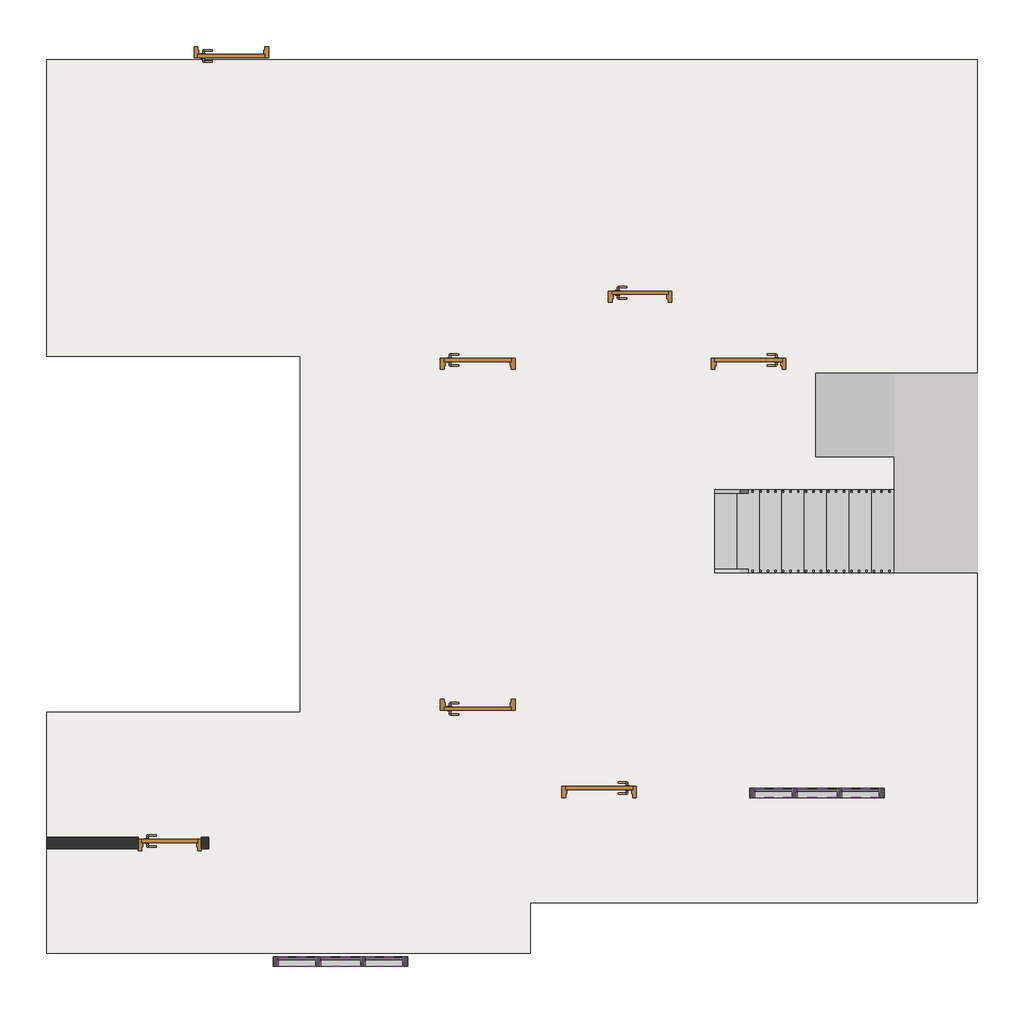
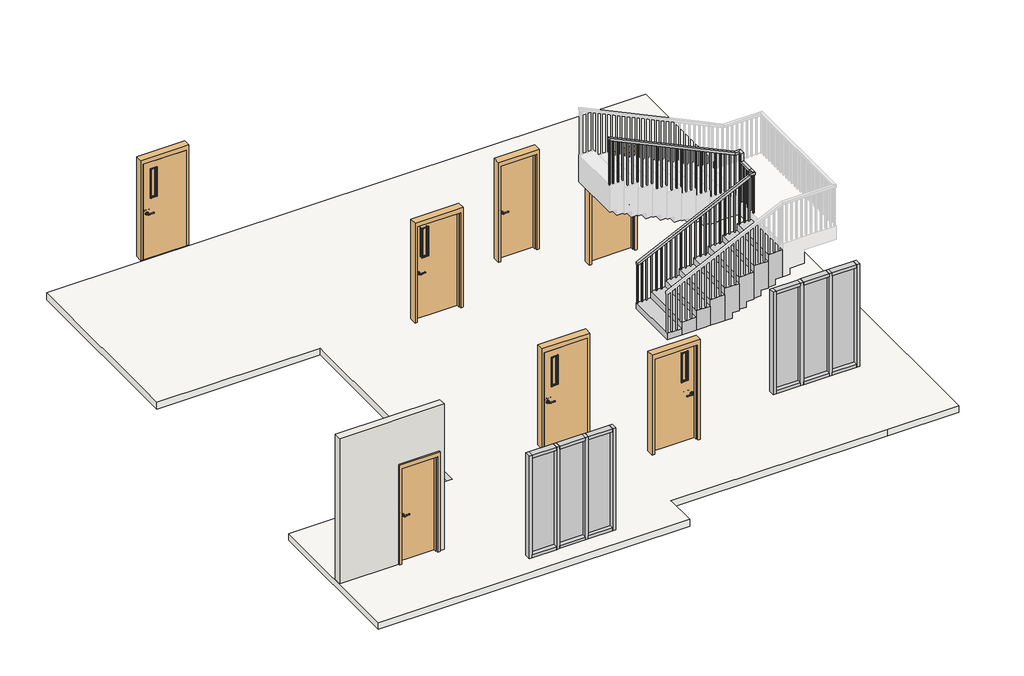
# One storey, part 1 of 2: 20 members, 7 doors, 6 plates, 1 railing, 1 slab, 1 stair flight, 1 wall.
"""IFC4 building model written with IfcOpenShell, lengths in millimetres."""

from ifc_helpers import new_model, si_unit, frame, origin, place, context, project, spatial, polyline, outline, extrude, faceted_brep, transform, mapped, element, save
from components import m_door_passage_single_flush_750_x_2000mm_a9826c90, m_door_passage_single_flush_750_x_2000mm_58848773, m_door_passage_single_vision_lite_900_x_2100_f7eb172f, m_door_passage_single_vision_lite_900_x_2100_15962226, rectangular_mullion_65_x_125mm_rectangular_c9dcdcb6, rectangular_mullion_65_x_125mm_rectangular_623ff0e3, rectangular_mullion_65_x_125mm_rectangular_3c6cccc9, rectangular_mullion_65_x_125mm_rectangular_2_9432af82, system_panel_glazed_03e68811, system_panel_glazed_7695abb4

model = new_model("IFC4")

# Units and contexts
model_context = context("Model", 3, world=origin())
ifc_project = project(units=[si_unit("LENGTHUNIT", "METRE", prefix="MILLI")], contexts=[model_context])

# Site, building, storey
site = spatial("IfcSite", under=ifc_project)
building = spatial("IfcBuilding", under=site)
storey = spatial("IfcBuildingStorey", under=building, Elevation=600.0)

# Doors
placement = place(None, origin())
m_door_passage_single_flush_750_x_2000mm_shape = m_door_passage_single_flush_750_x_2000mm_a9826c90(model_context)
element("IfcDoor", 1, ObjectType="M_Door-Passage-Single-Flush : 750 x 2000mm", at=placement, inside=storey, context=model_context, shape_type="MappedRepresentation", body=[
    mapped(m_door_passage_single_flush_750_x_2000mm_shape, transform((-18812.7520625, -8532.3980844, 600.0), x_axis=(1.0, 0.0, 0.0), y_axis=(0.0, 1.0, 0.0), z_axis=(0.0, 0.0, 1.0))),
])
m_door_passage_single_flush_750_x_2000mm_2_shape = m_door_passage_single_flush_750_x_2000mm_58848773(model_context)
element("IfcDoor", 2, ObjectType="M_Door-Passage-Single-Flush : 750 x 2000mm", at=placement, inside=storey, context=model_context, shape_type="MappedRepresentation", body=[
    mapped(m_door_passage_single_flush_750_x_2000mm_2_shape, transform((-12512.7520625, -1227.8980844, 600.0), x_axis=(1.0, 0.0, 0.0), y_axis=(0.0, 1.0, 0.0), z_axis=(0.0, 0.0, 1.0))),
])
m_door_passage_single_vision_lite_900_x_2100_shape = m_door_passage_single_vision_lite_900_x_2100_f7eb172f(model_context)
element("IfcDoor", 3, ObjectType="M_Door-Passage-Single-Vision_Lite : 900 x 2100", at=placement, inside=storey, context=model_context, shape_type="MappedRepresentation", body=[
    mapped(m_door_passage_single_vision_lite_900_x_2100_shape, transform((-13062.7520625, -7859.8980844, 600.0), x_axis=(-1.0, 0.0, 0.0), y_axis=(0.0, -1.0, 0.0), z_axis=(0.0, 0.0, 1.0))),
])
element("IfcDoor", 4, ObjectType="M_Door-Passage-Single-Vision_Lite : 900 x 2100", at=placement, inside=storey, context=model_context, shape_type="MappedRepresentation", body=[
    mapped(m_door_passage_single_vision_lite_900_x_2100_shape, transform((-11062.7520625, -2127.8980844, 600.0), x_axis=(-1.0, 0.0, 0.0), y_axis=(0.0, -1.0, 0.0), z_axis=(0.0, 0.0, 1.0))),
])
element("IfcDoor", 5, ObjectType="M_Door-Passage-Single-Vision_Lite : 900 x 2100", at=placement, inside=storey, context=model_context, shape_type="MappedRepresentation", body=[
    mapped(m_door_passage_single_vision_lite_900_x_2100_shape, transform((-14687.7520625, -6655.1980844, 600.0), x_axis=(1.0, 0.0, 0.0), y_axis=(0.0, 1.0, 0.0), z_axis=(0.0, 0.0, 1.0))),
])
element("IfcDoor", 6, ObjectType="M_Door-Passage-Single-Vision_Lite : 900 x 2100", at=placement, inside=storey, context=model_context, shape_type="MappedRepresentation", body=[
    mapped(m_door_passage_single_vision_lite_900_x_2100_shape, transform((-17987.7520625, 2084.8019156, 600.0), x_axis=(1.0, 0.0, 0.0), y_axis=(0.0, 1.0, 0.0), z_axis=(0.0, 0.0, 1.0))),
])
m_door_passage_single_vision_lite_900_x_2100_2_shape = m_door_passage_single_vision_lite_900_x_2100_15962226(model_context)
element("IfcDoor", 7, ObjectType="M_Door-Passage-Single-Vision_Lite : 900 x 2100", at=placement, inside=storey, context=model_context, shape_type="MappedRepresentation", body=[
    mapped(m_door_passage_single_vision_lite_900_x_2100_2_shape, transform((-14687.7520625, -2127.8980844, 600.0), x_axis=(1.0, 0.0, 0.0), y_axis=(0.0, 1.0, 0.0), z_axis=(0.0, 0.0, 1.0))),
])

# Members
rectangular_mullion_65_x_125mm_rectangular_shape = rectangular_mullion_65_x_125mm_rectangular_c9dcdcb6(model_context)
element("IfcMember", 8, ObjectType="Rectangular Mullion : 65 x 125mm rectangular", at=placement, inside=storey, context=model_context, shape_type="MappedRepresentation", body=[
    mapped(rectangular_mullion_65_x_125mm_rectangular_shape, transform((-15625.2520625, -10113.5480844, 1050.0), x_axis=(1.0, 0.0, 0.0), y_axis=(0.0, -1.0, 0.0), z_axis=(0.0, 0.0, -1.0))),
])
element("IfcMember", 9, ObjectType="Rectangular Mullion : 65 x 125mm rectangular", at=placement, inside=storey, context=model_context, shape_type="MappedRepresentation", body=[
    mapped(rectangular_mullion_65_x_125mm_rectangular_shape, transform((-9242.7520625, -7853.5480844, 1050.0), x_axis=(1.0, 0.0, 0.0), y_axis=(0.0, -1.0, 0.0), z_axis=(0.0, 0.0, -1.0))),
])
element("IfcMember", 10, ObjectType="Rectangular Mullion : 65 x 125mm rectangular", at=placement, inside=storey, context=model_context, shape_type="MappedRepresentation", body=[
    mapped(rectangular_mullion_65_x_125mm_rectangular_shape, transform((-17425.2520625, -10113.5480844, 3300.0), x_axis=(-1.0, 0.0, 0.0), y_axis=(0.0, -1.0, 0.0), z_axis=(0.0, 0.0, 1.0))),
])
element("IfcMember", 11, ObjectType="Rectangular Mullion : 65 x 125mm rectangular", at=placement, inside=storey, context=model_context, shape_type="MappedRepresentation", body=[
    mapped(rectangular_mullion_65_x_125mm_rectangular_shape, transform((-11042.7520625, -7853.5480844, 3300.0), x_axis=(-1.0, 0.0, 0.0), y_axis=(0.0, -1.0, 0.0), z_axis=(0.0, 0.0, 1.0))),
])
rectangular_mullion_65_x_125mm_rectangular_2_shape = rectangular_mullion_65_x_125mm_rectangular_623ff0e3(model_context)
element("IfcMember", 12, ObjectType="Rectangular Mullion : 65 x 125mm rectangular", at=placement, inside=storey, context=model_context, shape_type="MappedRepresentation", body=[
    mapped(rectangular_mullion_65_x_125mm_rectangular_2_shape, transform((-15690.2520625, -10113.5480844, 3300.0), x_axis=(0.0, 0.0, 1.0), y_axis=(0.0, -1.0, 0.0), z_axis=(1.0, 0.0, 0.0))),
])
element("IfcMember", 13, ObjectType="Rectangular Mullion : 65 x 125mm rectangular", at=placement, inside=storey, context=model_context, shape_type="MappedRepresentation", body=[
    mapped(rectangular_mullion_65_x_125mm_rectangular_2_shape, transform((-9307.7520625, -7853.5480844, 3300.0), x_axis=(0.0, 0.0, 1.0), y_axis=(0.0, -1.0, 0.0), z_axis=(1.0, 0.0, 0.0))),
])
element("IfcMember", 14, ObjectType="Rectangular Mullion : 65 x 125mm rectangular", at=placement, inside=storey, context=model_context, shape_type="MappedRepresentation", body=[
    mapped(rectangular_mullion_65_x_125mm_rectangular_2_shape, transform((-16857.7520625, -10113.5480844, 3300.0), x_axis=(0.0, 0.0, 1.0), y_axis=(0.0, -1.0, 0.0), z_axis=(1.0, 0.0, 0.0))),
])
element("IfcMember", 15, ObjectType="Rectangular Mullion : 65 x 125mm rectangular", at=placement, inside=storey, context=model_context, shape_type="MappedRepresentation", body=[
    mapped(rectangular_mullion_65_x_125mm_rectangular_2_shape, transform((-10475.2520625, -7853.5480844, 3300.0), x_axis=(0.0, 0.0, 1.0), y_axis=(0.0, -1.0, 0.0), z_axis=(1.0, 0.0, 0.0))),
])
element("IfcMember", 16, ObjectType="Rectangular Mullion : 65 x 125mm rectangular", at=placement, inside=storey, context=model_context, shape_type="MappedRepresentation", body=[
    mapped(rectangular_mullion_65_x_125mm_rectangular_2_shape, transform((-17360.2520625, -10113.5480844, 1050.0), x_axis=(0.0, 0.0, -1.0), y_axis=(0.0, -1.0, 0.0), z_axis=(-1.0, 0.0, 0.0))),
])
element("IfcMember", 17, ObjectType="Rectangular Mullion : 65 x 125mm rectangular", at=placement, inside=storey, context=model_context, shape_type="MappedRepresentation", body=[
    mapped(rectangular_mullion_65_x_125mm_rectangular_2_shape, transform((-10977.7520625, -7853.5480844, 1050.0), x_axis=(0.0, 0.0, -1.0), y_axis=(0.0, -1.0, 0.0), z_axis=(-1.0, 0.0, 0.0))),
])
element("IfcMember", 18, ObjectType="Rectangular Mullion : 65 x 125mm rectangular", at=placement, inside=storey, context=model_context, shape_type="MappedRepresentation", body=[
    mapped(rectangular_mullion_65_x_125mm_rectangular_2_shape, transform((-16192.7520625, -10113.5480844, 1050.0), x_axis=(0.0, 0.0, -1.0), y_axis=(0.0, -1.0, 0.0), z_axis=(-1.0, 0.0, 0.0))),
])
element("IfcMember", 19, ObjectType="Rectangular Mullion : 65 x 125mm rectangular", at=placement, inside=storey, context=model_context, shape_type="MappedRepresentation", body=[
    mapped(rectangular_mullion_65_x_125mm_rectangular_2_shape, transform((-9810.2520625, -7853.5480844, 1050.0), x_axis=(0.0, 0.0, -1.0), y_axis=(0.0, -1.0, 0.0), z_axis=(-1.0, 0.0, 0.0))),
])
rectangular_mullion_65_x_125mm_rectangular_3_shape = rectangular_mullion_65_x_125mm_rectangular_3c6cccc9(model_context)
element("IfcMember", 20, ObjectType="Rectangular Mullion : 65 x 125mm rectangular", at=placement, inside=storey, context=model_context, shape_type="MappedRepresentation", body=[
    mapped(rectangular_mullion_65_x_125mm_rectangular_3_shape, transform((-16792.7520625, -10113.5480844, 1050.0), x_axis=(0.0, 0.0, -1.0), y_axis=(0.0, -1.0, 0.0), z_axis=(-1.0, 0.0, 0.0))),
])
element("IfcMember", 21, ObjectType="Rectangular Mullion : 65 x 125mm rectangular", at=placement, inside=storey, context=model_context, shape_type="MappedRepresentation", body=[
    mapped(rectangular_mullion_65_x_125mm_rectangular_3_shape, transform((-10410.2520625, -7853.5480844, 1050.0), x_axis=(0.0, 0.0, -1.0), y_axis=(0.0, -1.0, 0.0), z_axis=(-1.0, 0.0, 0.0))),
])
element("IfcMember", 22, ObjectType="Rectangular Mullion : 65 x 125mm rectangular", at=placement, inside=storey, context=model_context, shape_type="MappedRepresentation", body=[
    mapped(rectangular_mullion_65_x_125mm_rectangular_3_shape, transform((-16257.7520625, -10113.5480844, 3300.0), x_axis=(0.0, 0.0, 1.0), y_axis=(0.0, -1.0, 0.0), z_axis=(1.0, 0.0, 0.0))),
])
element("IfcMember", 23, ObjectType="Rectangular Mullion : 65 x 125mm rectangular", at=placement, inside=storey, context=model_context, shape_type="MappedRepresentation", body=[
    mapped(rectangular_mullion_65_x_125mm_rectangular_3_shape, transform((-9875.2520625, -7853.5480844, 3300.0), x_axis=(0.0, 0.0, 1.0), y_axis=(0.0, -1.0, 0.0), z_axis=(1.0, 0.0, 0.0))),
])
rectangular_mullion_65_x_125mm_rectangular_2_2_shape = rectangular_mullion_65_x_125mm_rectangular_2_9432af82(model_context)
element("IfcMember", 24, ObjectType="Rectangular Mullion : 65 x 125mm rectangular 2", at=placement, inside=storey, context=model_context, shape_type="MappedRepresentation", body=[
    mapped(rectangular_mullion_65_x_125mm_rectangular_2_2_shape, transform((-10442.7520625, -7853.5480844, 1050.0), x_axis=(1.0, 0.0, 0.0), y_axis=(0.0, -1.0, 0.0), z_axis=(0.0, 0.0, -1.0))),
])
element("IfcMember", 25, ObjectType="Rectangular Mullion : 65 x 125mm rectangular 2", at=placement, inside=storey, context=model_context, shape_type="MappedRepresentation", body=[
    mapped(rectangular_mullion_65_x_125mm_rectangular_2_2_shape, transform((-9842.7520625, -7853.5480844, 1050.0), x_axis=(1.0, 0.0, 0.0), y_axis=(0.0, -1.0, 0.0), z_axis=(0.0, 0.0, -1.0))),
])
element("IfcMember", 26, ObjectType="Rectangular Mullion : 65 x 125mm rectangular 2", at=placement, inside=storey, context=model_context, shape_type="MappedRepresentation", body=[
    mapped(rectangular_mullion_65_x_125mm_rectangular_2_2_shape, transform((-16825.2520625, -10113.5480844, 1050.0), x_axis=(1.0, 0.0, 0.0), y_axis=(0.0, -1.0, 0.0), z_axis=(0.0, 0.0, -1.0))),
])
element("IfcMember", 27, ObjectType="Rectangular Mullion : 65 x 125mm rectangular 2", at=placement, inside=storey, context=model_context, shape_type="MappedRepresentation", body=[
    mapped(rectangular_mullion_65_x_125mm_rectangular_2_2_shape, transform((-16225.2520625, -10113.5480844, 1050.0), x_axis=(1.0, 0.0, 0.0), y_axis=(0.0, -1.0, 0.0), z_axis=(0.0, 0.0, -1.0))),
])

# Plates
system_panel_glazed_shape = system_panel_glazed_03e68811(model_context)
element("IfcPlate", 28, ObjectType="System Panel : Glazed", at=placement, inside=storey, context=model_context, shape_type="MappedRepresentation", body=[
    mapped(system_panel_glazed_shape, transform((-16525.2520625, -10113.5480844, 1115.0), x_axis=(1.0, 0.0, 0.0), y_axis=(0.0, 1.0, 0.0), z_axis=(0.0, 0.0, 1.0))),
])
element("IfcPlate", 29, ObjectType="System Panel : Glazed", at=placement, inside=storey, context=model_context, shape_type="MappedRepresentation", body=[
    mapped(system_panel_glazed_shape, transform((-10142.7520625, -7853.5480844, 1115.0), x_axis=(1.0, 0.0, 0.0), y_axis=(0.0, 1.0, 0.0), z_axis=(0.0, 0.0, 1.0))),
])
system_panel_glazed_2_shape = system_panel_glazed_7695abb4(model_context)
element("IfcPlate", 30, ObjectType="System Panel : Glazed", at=placement, inside=storey, context=model_context, shape_type="MappedRepresentation", body=[
    mapped(system_panel_glazed_2_shape, transform((-17109.0020625, -10113.5480844, 1115.0), x_axis=(1.0, 0.0, 0.0), y_axis=(0.0, 1.0, 0.0), z_axis=(0.0, 0.0, 1.0))),
])
element("IfcPlate", 31, ObjectType="System Panel : Glazed", at=placement, inside=storey, context=model_context, shape_type="MappedRepresentation", body=[
    mapped(system_panel_glazed_2_shape, transform((-10726.5020625, -7853.5480844, 1115.0), x_axis=(1.0, 0.0, 0.0), y_axis=(0.0, 1.0, 0.0), z_axis=(0.0, 0.0, 1.0))),
])
element("IfcPlate", 32, ObjectType="System Panel : Glazed", at=placement, inside=storey, context=model_context, shape_type="MappedRepresentation", body=[
    mapped(system_panel_glazed_2_shape, transform((-15941.5020625, -10113.5480844, 1115.0), x_axis=(1.0, 0.0, 0.0), y_axis=(0.0, 1.0, 0.0), z_axis=(0.0, 0.0, 1.0))),
])
element("IfcPlate", 33, ObjectType="System Panel : Glazed", at=placement, inside=storey, context=model_context, shape_type="MappedRepresentation", body=[
    mapped(system_panel_glazed_2_shape, transform((-9559.0020625, -7853.5480844, 1115.0), x_axis=(1.0, 0.0, 0.0), y_axis=(0.0, 1.0, 0.0), z_axis=(0.0, 0.0, 1.0))),
])

# Railing
element("IfcRailing", 34, ObjectType="Handrail - Rectangular", at=placement, inside=storey, context=model_context, shape_type="SolidModel", body=[
    faceted_brep([(-11513.3520625, -3791.8480844, 1642.1052632), (-11513.3520625, -3791.8480844, 1586.7794841), (-11513.3520625, -3841.8480844, 1586.7794841), (-11513.3520625, -3841.8480844, 1642.1052632), (-9187.9520625, -3791.8480844, 2743.6105263), (-9137.9520625, -3791.8480844, 2711.9689578), (-9137.9520625, -3841.8480844, 2711.9689578), (-9187.9520625, -3841.8480844, 2743.6105263), (-9187.9520625, -3791.8480844, 2778.9473684), (-9137.9520625, -3791.8480844, 2728.9473684), (-9137.9520625, -3841.8480844, 2728.9473684), (-9187.9520625, -3841.8480844, 2778.9473684), (-9112.9520625, -3791.8480844, 2778.9473684), (-9112.9520625, -3791.8480844, 2728.9473684), (-9062.9520625, -3841.8480844, 2728.9473684), (-9062.9520625, -3841.8480844, 2778.9473684), (-9112.9520625, -3716.8480844, 2778.9473684), (-9112.9520625, -3716.8480844, 2728.9473684), (-9062.9520625, -3716.8480844, 2728.9473684), (-9062.9520625, -3716.8480844, 2778.9473684), (-9112.9520625, -3426.2480844, 2778.9473684), (-9112.9520625, -3376.2480844, 2728.9473684), (-9062.9520625, -3376.2480844, 2728.9473684), (-9062.9520625, -3426.2480844, 2778.9473684), (-9112.9520625, -3426.2480844, 2956.3894737), (-9112.9520625, -3376.2480844, 2906.3894737), (-9062.9520625, -3376.2480844, 2906.3894737), (-9062.9520625, -3426.2480844, 2956.3894737), (-9112.9520625, -3351.2480844, 2956.3894737), (-9112.9520625, -3351.2480844, 2906.3894737), (-9062.9520625, -3301.2480844, 2906.3894737), (-9062.9520625, -3301.2480844, 2956.3894737), (-9187.9520625, -3351.2480844, 2956.3894737), (-9199.1953738, -3351.2480844, 2906.3894737), (-9199.1953738, -3301.2480844, 2906.3894737), (-9187.9520625, -3301.2480844, 2956.3894737), (-11813.3520625, -3351.2480844, 4200.0), (-11813.3520625, -3301.2480844, 4200.0), (-11813.3520625, -3301.2480844, 4144.6742209), (-11813.3520625, -3351.2480844, 4144.6742209)], [[[0, 1, 2, 3]], [[1, 0, 4, 5]], [[2, 1, 5, 6]], [[3, 2, 6, 7]], [[0, 3, 7, 4]], [[5, 4, 8, 9]], [[6, 5, 9, 10]], [[7, 6, 10, 11]], [[4, 7, 11, 8]], [[9, 8, 12, 13]], [[10, 9, 13, 14]], [[11, 10, 14, 15]], [[8, 11, 15, 12]], [[13, 12, 16, 17]], [[14, 13, 17, 18]], [[15, 14, 18, 19]], [[12, 15, 19, 16]], [[17, 16, 20, 21]], [[18, 17, 21, 22]], [[19, 18, 22, 23]], [[16, 19, 23, 20]], [[21, 20, 24, 25]], [[22, 21, 25, 26]], [[23, 22, 26, 27]], [[20, 23, 27, 24]], [[25, 24, 28, 29]], [[26, 25, 29, 30]], [[27, 26, 30, 31]], [[24, 27, 31, 28]], [[29, 28, 32, 33]], [[30, 29, 33, 34]], [[31, 30, 34, 35]], [[28, 31, 35, 32]], [[36, 37, 38, 39]], [[33, 32, 36, 39]], [[34, 33, 39, 38]], [[35, 34, 38, 37]], [[32, 35, 37, 36]]]),
    extrude(outline(polyline([(4100.242642, -11719.5520625), (4109.7163262, -11739.5520625), (3157.8947368, -11739.5520625), (3157.8947368, -11719.5520625), (4100.242642, -11719.5520625)])), frame((0.0, -3336.2480844, 0.0), z_axis=(0.0, 1.0, 0.0), x_axis=(0.0, 0.0, 1.0)), (0.0, 0.0, 1.0), 20.0),
    extrude(outline(polyline([(4052.1163262, -11617.9520625), (4061.5900104, -11637.9520625), (3157.8947368, -11637.9520625), (3157.8947368, -11617.9520625), (4052.1163262, -11617.9520625)])), frame((0.0, -3336.2480844, 0.0), z_axis=(0.0, 1.0, 0.0), x_axis=(0.0, 0.0, 1.0)), (0.0, 0.0, 1.0), 20.0),
    extrude(outline(polyline([(4003.9900104, -11516.3520625), (4013.4636946, -11536.3520625), (3157.8947368, -11536.3520625), (3157.8947368, -11516.3520625), (4003.9900104, -11516.3520625)])), frame((0.0, -3336.2480844, 0.0), z_axis=(0.0, 1.0, 0.0), x_axis=(0.0, 0.0, 1.0)), (0.0, 0.0, 1.0), 20.0),
    extrude(outline(polyline([(3955.8636946, -11414.7520625), (3965.3373788, -11434.7520625), (3015.7894737, -11434.7520625), (3015.7894737, -11414.7520625), (3955.8636946, -11414.7520625)])), frame((0.0, -3336.2480844, 0.0), z_axis=(0.0, 1.0, 0.0), x_axis=(0.0, 0.0, 1.0)), (0.0, 0.0, 1.0), 20.0),
    extrude(outline(polyline([(3907.7373788, -11313.1520625), (3917.211063, -11333.1520625), (3015.7894737, -11333.1520625), (3015.7894737, -11313.1520625), (3907.7373788, -11313.1520625)])), frame((0.0, -3336.2480844, 0.0), z_axis=(0.0, 1.0, 0.0), x_axis=(0.0, 0.0, 1.0)), (0.0, 0.0, 1.0), 20.0),
    extrude(outline(polyline([(3859.611063, -11211.5520625), (3869.0847473, -11231.5520625), (3015.7894737, -11231.5520625), (3015.7894737, -11211.5520625), (3859.611063, -11211.5520625)])), frame((0.0, -3336.2480844, 0.0), z_axis=(0.0, 1.0, 0.0), x_axis=(0.0, 0.0, 1.0)), (0.0, 0.0, 1.0), 20.0),
    extrude(outline(polyline([(3811.4847473, -11109.9520625), (3820.9584315, -11129.9520625), (2873.6842105, -11129.9520625), (2873.6842105, -11109.9520625), (3811.4847473, -11109.9520625)])), frame((0.0, -3336.2480844, 0.0), z_axis=(0.0, 1.0, 0.0), x_axis=(0.0, 0.0, 1.0)), (0.0, 0.0, 1.0), 20.0),
    extrude(outline(polyline([(3763.3584315, -11008.3520625), (3772.8321157, -11028.3520625), (2873.6842105, -11028.3520625), (2873.6842105, -11008.3520625), (3763.3584315, -11008.3520625)])), frame((0.0, -3336.2480844, 0.0), z_axis=(0.0, 1.0, 0.0), x_axis=(0.0, 0.0, 1.0)), (0.0, 0.0, 1.0), 20.0),
    extrude(outline(polyline([(3715.2321157, -10906.7520625), (3724.7057999, -10926.7520625), (2873.6842105, -10926.7520625), (2873.6842105, -10906.7520625), (3715.2321157, -10906.7520625)])), frame((0.0, -3336.2480844, 0.0), z_axis=(0.0, 1.0, 0.0), x_axis=(0.0, 0.0, 1.0)), (0.0, 0.0, 1.0), 20.0),
    extrude(outline(polyline([(3667.1057999, -10805.1520625), (3676.5794841, -10825.1520625), (2731.5789474, -10825.1520625), (2731.5789474, -10805.1520625), (3667.1057999, -10805.1520625)])), frame((0.0, -3336.2480844, 0.0), z_axis=(0.0, 1.0, 0.0), x_axis=(0.0, 0.0, 1.0)), (0.0, 0.0, 1.0), 20.0),
    extrude(outline(polyline([(3618.9794841, -10703.5520625), (3628.4531683, -10723.5520625), (2731.5789474, -10723.5520625), (2731.5789474, -10703.5520625), (3618.9794841, -10703.5520625)])), frame((0.0, -3336.2480844, 0.0), z_axis=(0.0, 1.0, 0.0), x_axis=(0.0, 0.0, 1.0)), (0.0, 0.0, 1.0), 20.0),
    extrude(outline(polyline([(3570.8531683, -10601.9520625), (3580.3268525, -10621.9520625), (2589.4736842, -10621.9520625), (2589.4736842, -10601.9520625), (3570.8531683, -10601.9520625)])), frame((0.0, -3336.2480844, 0.0), z_axis=(0.0, 1.0, 0.0), x_axis=(0.0, 0.0, 1.0)), (0.0, 0.0, 1.0), 20.0),
    extrude(outline(polyline([(3522.7268525, -10500.3520625), (3532.2005367, -10520.3520625), (2589.4736842, -10520.3520625), (2589.4736842, -10500.3520625), (3522.7268525, -10500.3520625)])), frame((0.0, -3336.2480844, 0.0), z_axis=(0.0, 1.0, 0.0), x_axis=(0.0, 0.0, 1.0)), (0.0, 0.0, 1.0), 20.0),
    extrude(outline(polyline([(3474.6005367, -10398.7520625), (3484.0742209, -10418.7520625), (2589.4736842, -10418.7520625), (2589.4736842, -10398.7520625), (3474.6005367, -10398.7520625)])), frame((0.0, -3336.2480844, 0.0), z_axis=(0.0, 1.0, 0.0), x_axis=(0.0, 0.0, 1.0)), (0.0, 0.0, 1.0), 20.0),
    extrude(outline(polyline([(3426.4742209, -10297.1520625), (3435.9479052, -10317.1520625), (2447.3684211, -10317.1520625), (2447.3684211, -10297.1520625), (3426.4742209, -10297.1520625)])), frame((0.0, -3336.2480844, 0.0), z_axis=(0.0, 1.0, 0.0), x_axis=(0.0, 0.0, 1.0)), (0.0, 0.0, 1.0), 20.0),
    extrude(outline(polyline([(3378.3479052, -10195.5520625), (3387.8215894, -10215.5520625), (2447.3684211, -10215.5520625), (2447.3684211, -10195.5520625), (3378.3479052, -10195.5520625)])), frame((0.0, -3336.2480844, 0.0), z_axis=(0.0, 1.0, 0.0), x_axis=(0.0, 0.0, 1.0)), (0.0, 0.0, 1.0), 20.0),
    extrude(outline(polyline([(3330.2215894, -10093.9520625), (3339.6952736, -10113.9520625), (2447.3684211, -10113.9520625), (2447.3684211, -10093.9520625), (3330.2215894, -10093.9520625)])), frame((0.0, -3336.2480844, 0.0), z_axis=(0.0, 1.0, 0.0), x_axis=(0.0, 0.0, 1.0)), (0.0, 0.0, 1.0), 20.0),
    extrude(outline(polyline([(3282.0952736, -9992.3520625), (3291.5689578, -10012.3520625), (2305.2631579, -10012.3520625), (2305.2631579, -9992.3520625), (3282.0952736, -9992.3520625)])), frame((0.0, -3336.2480844, 0.0), z_axis=(0.0, 1.0, 0.0), x_axis=(0.0, 0.0, 1.0)), (0.0, 0.0, 1.0), 20.0),
    extrude(outline(polyline([(3233.9689578, -9890.7520625), (3243.442642, -9910.7520625), (2305.2631579, -9910.7520625), (2305.2631579, -9890.7520625), (3233.9689578, -9890.7520625)])), frame((0.0, -3336.2480844, 0.0), z_axis=(0.0, 1.0, 0.0), x_axis=(0.0, 0.0, 1.0)), (0.0, 0.0, 1.0), 20.0),
    extrude(outline(polyline([(3185.842642, -9789.1520625), (3195.3163262, -9809.1520625), (2305.2631579, -9809.1520625), (2305.2631579, -9789.1520625), (3185.842642, -9789.1520625)])), frame((0.0, -3336.2480844, 0.0), z_axis=(0.0, 1.0, 0.0), x_axis=(0.0, 0.0, 1.0)), (0.0, 0.0, 1.0), 20.0),
    extrude(outline(polyline([(3137.7163262, -9687.5520625), (3147.1900104, -9707.5520625), (2163.1578947, -9707.5520625), (2163.1578947, -9687.5520625), (3137.7163262, -9687.5520625)])), frame((0.0, -3336.2480844, 0.0), z_axis=(0.0, 1.0, 0.0), x_axis=(0.0, 0.0, 1.0)), (0.0, 0.0, 1.0), 20.0),
    extrude(outline(polyline([(3089.5900104, -9585.9520625), (3099.0636946, -9605.9520625), (2163.1578947, -9605.9520625), (2163.1578947, -9585.9520625), (3089.5900104, -9585.9520625)])), frame((0.0, -3336.2480844, 0.0), z_axis=(0.0, 1.0, 0.0), x_axis=(0.0, 0.0, 1.0)), (0.0, 0.0, 1.0), 20.0),
    extrude(outline(polyline([(3041.4636946, -9484.3520625), (3050.9373788, -9504.3520625), (2163.1578947, -9504.3520625), (2163.1578947, -9484.3520625), (3041.4636946, -9484.3520625)])), frame((0.0, -3336.2480844, 0.0), z_axis=(0.0, 1.0, 0.0), x_axis=(0.0, 0.0, 1.0)), (0.0, 0.0, 1.0), 20.0),
    extrude(outline(polyline([(2993.3373788, -9382.7520625), (3002.811063, -9402.7520625), (2021.0526316, -9402.7520625), (2021.0526316, -9382.7520625), (2993.3373788, -9382.7520625)])), frame((0.0, -3336.2480844, 0.0), z_axis=(0.0, 1.0, 0.0), x_axis=(0.0, 0.0, 1.0)), (0.0, 0.0, 1.0), 20.0),
    extrude(outline(polyline([(2945.211063, -9281.1520625), (2954.6847473, -9301.1520625), (2021.0526316, -9301.1520625), (2021.0526316, -9281.1520625), (2945.211063, -9281.1520625)])), frame((0.0, -3336.2480844, 0.0), z_axis=(0.0, 1.0, 0.0), x_axis=(0.0, 0.0, 1.0)), (0.0, 0.0, 1.0), 20.0),
    extrude(outline(polyline([(2897.0847473, -9179.5520625), (2906.5584315, -9199.5520625), (2021.0526316, -9199.5520625), (2021.0526316, -9179.5520625), (2897.0847473, -9179.5520625)])), frame((0.0, -3336.2480844, 0.0), z_axis=(0.0, 1.0, 0.0), x_axis=(0.0, 0.0, 1.0)), (0.0, 0.0, 1.0), 20.0),
    extrude(outline(polyline([(-9097.9520625, -3420.4480844), (-9097.9520625, -3400.4480844), (-9077.9520625, -3400.4480844), (-9077.9520625, -3420.4480844), (-9097.9520625, -3420.4480844)])), frame((0.0, 0.0, 1878.9473684), z_axis=(0.0, 0.0, 1.0), x_axis=(1.0, 0.0, 0.0)), (0.0, 0.0, 1.0), 1027.4421053),
    extrude(outline(polyline([(-9097.9520625, -3522.0480844), (-9097.9520625, -3502.0480844), (-9077.9520625, -3502.0480844), (-9077.9520625, -3522.0480844), (-9097.9520625, -3522.0480844)])), frame((0.0, 0.0, 1878.9473684), z_axis=(0.0, 0.0, 1.0), x_axis=(1.0, 0.0, 0.0)), (0.0, 0.0, 1.0), 850.0),
    extrude(outline(polyline([(-9097.9520625, -3623.6480844), (-9097.9520625, -3603.6480844), (-9077.9520625, -3603.6480844), (-9077.9520625, -3623.6480844), (-9097.9520625, -3623.6480844)])), frame((0.0, 0.0, 1878.9473684), z_axis=(0.0, 0.0, 1.0), x_axis=(1.0, 0.0, 0.0)), (0.0, 0.0, 1.0), 850.0),
    extrude(outline(polyline([(-9097.9520625, -3725.2480844), (-9097.9520625, -3705.2480844), (-9077.9520625, -3705.2480844), (-9077.9520625, -3725.2480844), (-9097.9520625, -3725.2480844)])), frame((0.0, 0.0, 1878.9473684), z_axis=(0.0, 0.0, 1.0), x_axis=(1.0, 0.0, 0.0)), (0.0, 0.0, 1.0), 850.0),
    extrude(outline(polyline([(-9186.5520625, -3806.8480844), (-9166.5520625, -3806.8480844), (-9166.5520625, -3826.8480844), (-9186.5520625, -3826.8480844), (-9186.5520625, -3806.8480844)])), frame((0.0, 0.0, 1736.8421053), z_axis=(0.0, 0.0, 1.0), x_axis=(1.0, 0.0, 0.0)), (0.0, 0.0, 1.0), 992.1052632),
    extrude(outline(polyline([(1736.8421053, -9288.1520625), (1736.8421053, -9268.1520625), (2650.2952736, -9268.1520625), (2640.8215894, -9288.1520625), (1736.8421053, -9288.1520625)])), frame((0.0, -3826.8480844, 0.0), z_axis=(0.0, 1.0, 0.0), x_axis=(0.0, 0.0, 1.0)), (0.0, 0.0, 1.0), 20.0),
    extrude(outline(polyline([(1736.8421053, -9389.7520625), (1736.8421053, -9369.7520625), (2602.1689578, -9369.7520625), (2592.6952736, -9389.7520625), (1736.8421053, -9389.7520625)])), frame((0.0, -3826.8480844, 0.0), z_axis=(0.0, 1.0, 0.0), x_axis=(0.0, 0.0, 1.0)), (0.0, 0.0, 1.0), 20.0),
    extrude(outline(polyline([(1594.7368421, -9491.3520625), (1594.7368421, -9471.3520625), (2554.042642, -9471.3520625), (2544.5689578, -9491.3520625), (1594.7368421, -9491.3520625)])), frame((0.0, -3826.8480844, 0.0), z_axis=(0.0, 1.0, 0.0), x_axis=(0.0, 0.0, 1.0)), (0.0, 0.0, 1.0), 20.0),
    extrude(outline(polyline([(1594.7368421, -9592.9520625), (1594.7368421, -9572.9520625), (2505.9163262, -9572.9520625), (2496.442642, -9592.9520625), (1594.7368421, -9592.9520625)])), frame((0.0, -3826.8480844, 0.0), z_axis=(0.0, 1.0, 0.0), x_axis=(0.0, 0.0, 1.0)), (0.0, 0.0, 1.0), 20.0),
    extrude(outline(polyline([(1594.7368421, -9694.5520625), (1594.7368421, -9674.5520625), (2457.7900104, -9674.5520625), (2448.3163262, -9694.5520625), (1594.7368421, -9694.5520625)])), frame((0.0, -3826.8480844, 0.0), z_axis=(0.0, 1.0, 0.0), x_axis=(0.0, 0.0, 1.0)), (0.0, 0.0, 1.0), 20.0),
    extrude(outline(polyline([(1452.6315789, -9796.1520625), (1452.6315789, -9776.1520625), (2409.6636946, -9776.1520625), (2400.1900104, -9796.1520625), (1452.6315789, -9796.1520625)])), frame((0.0, -3826.8480844, 0.0), z_axis=(0.0, 1.0, 0.0), x_axis=(0.0, 0.0, 1.0)), (0.0, 0.0, 1.0), 20.0),
    extrude(outline(polyline([(1452.6315789, -9897.7520625), (1452.6315789, -9877.7520625), (2361.5373788, -9877.7520625), (2352.0636946, -9897.7520625), (1452.6315789, -9897.7520625)])), frame((0.0, -3826.8480844, 0.0), z_axis=(0.0, 1.0, 0.0), x_axis=(0.0, 0.0, 1.0)), (0.0, 0.0, 1.0), 20.0),
    extrude(outline(polyline([(1452.6315789, -9999.3520625), (1452.6315789, -9979.3520625), (2313.411063, -9979.3520625), (2303.9373788, -9999.3520625), (1452.6315789, -9999.3520625)])), frame((0.0, -3826.8480844, 0.0), z_axis=(0.0, 1.0, 0.0), x_axis=(0.0, 0.0, 1.0)), (0.0, 0.0, 1.0), 20.0),
    extrude(outline(polyline([(1310.5263158, -10100.9520625), (1310.5263158, -10080.9520625), (2265.2847473, -10080.9520625), (2255.811063, -10100.9520625), (1310.5263158, -10100.9520625)])), frame((0.0, -3826.8480844, 0.0), z_axis=(0.0, 1.0, 0.0), x_axis=(0.0, 0.0, 1.0)), (0.0, 0.0, 1.0), 20.0),
    extrude(outline(polyline([(1310.5263158, -10202.5520625), (1310.5263158, -10182.5520625), (2217.1584315, -10182.5520625), (2207.6847473, -10202.5520625), (1310.5263158, -10202.5520625)])), frame((0.0, -3826.8480844, 0.0), z_axis=(0.0, 1.0, 0.0), x_axis=(0.0, 0.0, 1.0)), (0.0, 0.0, 1.0), 20.0),
    extrude(outline(polyline([(1310.5263158, -10304.1520625), (1310.5263158, -10284.1520625), (2169.0321157, -10284.1520625), (2159.5584315, -10304.1520625), (1310.5263158, -10304.1520625)])), frame((0.0, -3826.8480844, 0.0), z_axis=(0.0, 1.0, 0.0), x_axis=(0.0, 0.0, 1.0)), (0.0, 0.0, 1.0), 20.0),
    extrude(outline(polyline([(1168.4210526, -10405.7520625), (1168.4210526, -10385.7520625), (2120.9057999, -10385.7520625), (2111.4321157, -10405.7520625), (1168.4210526, -10405.7520625)])), frame((0.0, -3826.8480844, 0.0), z_axis=(0.0, 1.0, 0.0), x_axis=(0.0, 0.0, 1.0)), (0.0, 0.0, 1.0), 20.0),
    extrude(outline(polyline([(1168.4210526, -10507.3520625), (1168.4210526, -10487.3520625), (2072.7794841, -10487.3520625), (2063.3057999, -10507.3520625), (1168.4210526, -10507.3520625)])), frame((0.0, -3826.8480844, 0.0), z_axis=(0.0, 1.0, 0.0), x_axis=(0.0, 0.0, 1.0)), (0.0, 0.0, 1.0), 20.0),
    extrude(outline(polyline([(1168.4210526, -10608.9520625), (1168.4210526, -10588.9520625), (2024.6531683, -10588.9520625), (2015.1794841, -10608.9520625), (1168.4210526, -10608.9520625)])), frame((0.0, -3826.8480844, 0.0), z_axis=(0.0, 1.0, 0.0), x_axis=(0.0, 0.0, 1.0)), (0.0, 0.0, 1.0), 20.0),
    extrude(outline(polyline([(1026.3157895, -10710.5520625), (1026.3157895, -10690.5520625), (1976.5268525, -10690.5520625), (1967.0531683, -10710.5520625), (1026.3157895, -10710.5520625)])), frame((0.0, -3826.8480844, 0.0), z_axis=(0.0, 1.0, 0.0), x_axis=(0.0, 0.0, 1.0)), (0.0, 0.0, 1.0), 20.0),
    extrude(outline(polyline([(1026.3157895, -10812.1520625), (1026.3157895, -10792.1520625), (1928.4005367, -10792.1520625), (1918.9268525, -10812.1520625), (1026.3157895, -10812.1520625)])), frame((0.0, -3826.8480844, 0.0), z_axis=(0.0, 1.0, 0.0), x_axis=(0.0, 0.0, 1.0)), (0.0, 0.0, 1.0), 20.0),
    extrude(outline(polyline([(1026.3157895, -10913.7520625), (1026.3157895, -10893.7520625), (1880.2268525, -10893.7520625), (1870.7531683, -10913.7520625), (1026.3157895, -10913.7520625)])), frame((0.0, -3826.8480844, 0.0), z_axis=(0.0, 1.0, 0.0), x_axis=(0.0, 0.0, 1.0)), (0.0, 0.0, 1.0), 20.0),
    extrude(outline(polyline([(884.2105263, -11015.3520625), (884.2105263, -10995.3520625), (1832.1479052, -10995.3520625), (1822.6742209, -11015.3520625), (884.2105263, -11015.3520625)])), frame((0.0, -3826.8480844, 0.0), z_axis=(0.0, 1.0, 0.0), x_axis=(0.0, 0.0, 1.0)), (0.0, 0.0, 1.0), 20.0),
    extrude(outline(polyline([(884.2105263, -11116.9520625), (884.2105263, -11096.9520625), (1784.0215894, -11096.9520625), (1774.5479052, -11116.9520625), (884.2105263, -11116.9520625)])), frame((0.0, -3826.8480844, 0.0), z_axis=(0.0, 1.0, 0.0), x_axis=(0.0, 0.0, 1.0)), (0.0, 0.0, 1.0), 20.0),
    extrude(outline(polyline([(884.2105263, -11218.5520625), (884.2105263, -11198.5520625), (1735.8952736, -11198.5520625), (1726.4215894, -11218.5520625), (884.2105263, -11218.5520625)])), frame((0.0, -3826.8480844, 0.0), z_axis=(0.0, 1.0, 0.0), x_axis=(0.0, 0.0, 1.0)), (0.0, 0.0, 1.0), 20.0),
    extrude(outline(polyline([(742.1052632, -11320.1520625), (742.1052632, -11300.1520625), (1687.7689578, -11300.1520625), (1678.2952736, -11320.1520625), (742.1052632, -11320.1520625)])), frame((0.0, -3826.8480844, 0.0), z_axis=(0.0, 1.0, 0.0), x_axis=(0.0, 0.0, 1.0)), (0.0, 0.0, 1.0), 20.0),
    extrude(outline(polyline([(742.1052632, -11421.7520625), (742.1052632, -11401.7520625), (1639.642642, -11401.7520625), (1630.1689578, -11421.7520625), (742.1052632, -11421.7520625)])), frame((0.0, -3826.8480844, 0.0), z_axis=(0.0, 1.0, 0.0), x_axis=(0.0, 0.0, 1.0)), (0.0, 0.0, 1.0), 20.0),
    extrude(outline(polyline([(-9097.9520625, -3336.2480844), (-9097.9520625, -3316.2480844), (-9077.9520625, -3316.2480844), (-9077.9520625, -3336.2480844), (-9097.9520625, -3336.2480844)])), frame((0.0, 0.0, 1878.9473684), z_axis=(0.0, 0.0, 1.0), x_axis=(1.0, 0.0, 0.0)), (0.0, 0.0, 1.0), 1027.4421053),
    extrude(outline(polyline([(-9097.9520625, -3806.8480844), (-9077.9520625, -3806.8480844), (-9077.9520625, -3826.8480844), (-9097.9520625, -3826.8480844), (-9097.9520625, -3806.8480844)])), frame((0.0, 0.0, 1878.9473684), z_axis=(0.0, 0.0, 1.0), x_axis=(1.0, 0.0, 0.0)), (0.0, 0.0, 1.0), 850.0),
    extrude(outline(polyline([(4135.4373788, -11793.8520625), (4144.911063, -11813.8520625), (3157.8947368, -11813.8520625), (3157.8947368, -11793.8520625), (4135.4373788, -11793.8520625)])), frame((0.0, -3336.2480844, 0.0), z_axis=(0.0, 1.0, 0.0), x_axis=(0.0, 0.0, 1.0)), (0.0, 0.0, 1.0), 20.0),
    extrude(outline(polyline([(742.1052632, -11513.8520625), (742.1052632, -11493.8520625), (1596.0163262, -11493.8520625), (1586.542642, -11513.8520625), (742.1052632, -11513.8520625)])), frame((0.0, -3826.8480844, 0.0), z_axis=(0.0, 1.0, 0.0), x_axis=(0.0, 0.0, 1.0)), (0.0, 0.0, 1.0), 20.0),
])

# Slab
element("IfcSlab", 35, ObjectType="01-150 floor", at=placement, inside=storey, context=model_context, shape_type="SweptSolid", body=[
    extrude(outline(polyline([(-7995.7520625, 1965.9519156), (-7995.7520625, -9326.0480844), (-9470.7520625, -9326.0480844), (-13987.7520625, -9326.0480844), (-13987.7520625, -10001.0480844), (-20462.7520625, -10001.0480844), (-20462.7520625, -6774.0480844), (-17062.7520625, -6774.0480844), (-17062.7520625, -2009.0480844), (-20462.7520625, -2009.0480844), (-20462.7520625, 1965.9519156), (-7995.7520625, 1965.9519156)])), frame((0.0, 0.0, 450.0), z_axis=(0.0, 0.0, 1.0), x_axis=(1.0, 0.0, 0.0)), (0.0, 0.0, 1.0), 150.0),
])

# Stair flight
element("IfcStairFlight", 36, ObjectType="M_Monolithic Run", at=placement, inside=storey, context=model_context, shape_type="Brep", body=[
    faceted_brep([(-11213.3520625, -3791.4480844, 742.1052632), (-11513.3520625, -3791.4480844, 742.1052632), (-11513.3520625, -4909.0480844, 742.1052632), (-11213.3520625, -4909.0480844, 742.1052632), (-11213.3520625, -3791.4480844, 600.0), (-11513.3520625, -3791.4480844, 600.0), (-11513.3520625, -4909.0480844, 600.0), (-11213.3520625, -4909.0480844, 600.0), (-10913.3520625, -3791.4480844, 884.2105263), (-11213.3520625, -3791.4480844, 884.2105263), (-11213.3520625, -4909.0480844, 884.2105263), (-10913.3520625, -4909.0480844, 884.2105263), (-10913.3520625, -3791.4480844, 600.0), (-10913.3520625, -4909.0480844, 600.0), (-10613.3520625, -3791.4480844, 1026.3157895), (-10913.3520625, -3791.4480844, 1026.3157895), (-10913.3520625, -4909.0480844, 1026.3157895), (-10613.3520625, -4909.0480844, 1026.3157895), (-10613.3520625, -3791.4480844, 600.0), (-10613.3520625, -4909.0480844, 600.0), (-10313.3520625, -3791.4480844, 1168.4210526), (-10613.3520625, -3791.4480844, 1168.4210526), (-10613.3520625, -4909.0480844, 1168.4210526), (-10313.3520625, -4909.0480844, 1168.4210526), (-10313.3520625, -3791.4480844, 600.0), (-10313.3520625, -4909.0480844, 600.0), (-10013.3520625, -3791.4480844, 1310.5263158), (-10313.3520625, -3791.4480844, 1310.5263158), (-10313.3520625, -4909.0480844, 1310.5263158), (-10013.3520625, -4909.0480844, 1310.5263158), (-10013.3520625, -3791.4480844, 742.1052632), (-10013.3520625, -3791.4480844, 718.4210526), (-10163.3520625, -3791.4480844, 718.4210526), (-10163.3520625, -3791.4480844, 600.0), (-10163.3520625, -4909.0480844, 600.0), (-10163.3520625, -4909.0480844, 718.4210526), (-10013.3520625, -4909.0480844, 718.4210526), (-10013.3520625, -4909.0480844, 742.1052632), (-9713.3520625, -3791.4480844, 1452.6315789), (-10013.3520625, -3791.4480844, 1452.6315789), (-10013.3520625, -4909.0480844, 1452.6315789), (-9713.3520625, -4909.0480844, 1452.6315789), (-9863.3520625, -3791.4480844, 742.1052632), (-9863.3520625, -4909.0480844, 742.1052632), (-9713.3520625, -3791.4480844, 884.2105263), (-9713.3520625, -3791.4480844, 860.5263158), (-9863.3520625, -3791.4480844, 860.5263158), (-9863.3520625, -4909.0480844, 860.5263158), (-9713.3520625, -4909.0480844, 860.5263158), (-9713.3520625, -4909.0480844, 884.2105263), (-9413.3520625, -3791.4480844, 1594.7368421), (-9713.3520625, -3791.4480844, 1594.7368421), (-9713.3520625, -4909.0480844, 1594.7368421), (-9413.3520625, -4909.0480844, 1594.7368421), (-9563.3520625, -3791.4480844, 884.2105263), (-9563.3520625, -4909.0480844, 884.2105263), (-9413.3520625, -3791.4480844, 1026.3157895), (-9413.3520625, -3791.4480844, 1002.6315789), (-9563.3520625, -3791.4480844, 1002.6315789), (-9563.3520625, -4909.0480844, 1002.6315789), (-9413.3520625, -4909.0480844, 1002.6315789), (-9413.3520625, -4909.0480844, 1026.3157895), (-9113.3520625, -3791.4480844, 1736.8421053), (-9413.3520625, -3791.4480844, 1736.8421053), (-9413.3520625, -4909.0480844, 1736.8421053), (-9113.3520625, -4909.0480844, 1736.8421053), (-9263.3520625, -3791.4480844, 1026.3157895), (-9263.3520625, -4909.0480844, 1026.3157895), (-9113.3520625, -3791.4480844, 1578.9473684), (-9113.3520625, -3791.4480844, 1144.7368421), (-9263.3520625, -3791.4480844, 1144.7368421), (-9263.3520625, -4909.0480844, 1144.7368421), (-9113.3520625, -4909.0480844, 1144.7368421)], [[[0, 1, 2, 3]], [[1, 0, 4, 5]], [[2, 1, 5, 6]], [[3, 2, 6, 7]], [[8, 9, 10, 11]], [[4, 0, 9, 8, 12]], [[0, 3, 10, 9]], [[3, 7, 13, 11, 10]], [[14, 15, 16, 17]], [[12, 8, 15, 14, 18]], [[8, 11, 16, 15]], [[11, 13, 19, 17, 16]], [[20, 21, 22, 23]], [[18, 14, 21, 20, 24]], [[14, 17, 22, 21]], [[17, 19, 25, 23, 22]], [[26, 27, 28, 29]], [[24, 20, 27, 26, 30, 31, 32, 33]], [[20, 23, 28, 27]], [[23, 25, 34, 35, 36, 37, 29, 28]], [[30, 37, 36, 31]], [[38, 39, 40, 41]], [[37, 30, 42, 43]], [[30, 26, 39, 38, 44, 45, 46, 42]], [[26, 29, 40, 39]], [[29, 37, 43, 47, 48, 49, 41, 40]], [[44, 49, 48, 45]], [[50, 51, 52, 53]], [[49, 44, 54, 55]], [[44, 38, 51, 50, 56, 57, 58, 54]], [[38, 41, 52, 51]], [[41, 49, 55, 59, 60, 61, 53, 52]], [[56, 61, 60, 57]], [[62, 63, 64, 65]], [[61, 56, 66, 67]], [[56, 50, 63, 62, 68, 69, 70, 66]], [[50, 53, 64, 63]], [[53, 61, 67, 71, 72, 65, 64]], [[62, 65, 72, 69, 68]], [[5, 4, 12, 18, 24, 33, 34, 25, 19, 13, 7, 6]], [[32, 35, 34, 33]], [[35, 32, 31, 36]], [[46, 47, 43, 42]], [[47, 46, 45, 48]], [[58, 59, 55, 54]], [[59, 58, 57, 60]], [[70, 71, 67, 66]], [[71, 70, 69, 72]]]),
])

# Wall
element("IfcWall", 37, ObjectType="02-150 wall", at=placement, inside=storey, context=model_context, shape_type="SweptSolid", body=[
    extrude(outline(polyline([(3800.0, -18287.7520625), (3800.0, -20462.7520625), (600.0, -20462.7520625), (600.0, -19237.7520625), (2800.0, -19237.7520625), (2800.0, -18387.7520625), (600.0, -18387.7520625), (600.0, -18287.7520625), (3800.0, -18287.7520625)])), frame((0.0, -8601.0480844, 0.0), z_axis=(0.0, 1.0, 0.0), x_axis=(0.0, 0.0, 1.0)), (0.0, 0.0, 1.0), 150.0),
])

save(model, "model.ifc")

# Revit data of these elements
# Type "M_Door-Passage-Single-Flush : 750 x 2000mm"
#   Type Mark = "35"
#   Assembly Code = "B2030200"
#   Analytic Construction = "Wooden"
#   Thickness = 45 mm
#   Thermal Resistance (R) = 0.455703 (m²·K)/W
#   Swing Angle [instance default] = 90.00°
#   Strike Height = 1000 mm
#   Rough Width [instance default] = 850 mm
#   Rough Height [instance default] = 2200 mm
#   MF Opening Height [instance default] = 100 mm
#   MF Opening Width [instance default] = 100 mm
#   Inset Calculate [instance default] = 105 mm
#   Masonry Inset [instance default] = 25 mm
#   Height = 2100 mm
#   Width = 750 mm
#   Heat Transfer Coefficient (U) = 2.19465 W/(m²·K)
#   Masonry Frame Depth = 150 mm
#   Masonry Frame [instance default] = yes
#   Function = 1
#   Dry Wall Frame [instance default] = no
#   Panel Material = Wood - Birch
#   Frame Material = Metal - Paint Finish - Grey
#   Door Handle Material = Aluminum
#   Visual Light Transmittance = 0
#   Solar Heat Gain Coefficient = 0
#   Wall Closure = (empty or 0)
# Type "M_Door-Passage-Single-Vision_Lite : 900 x 2100"
#   Type Mark = "46"
#   Assembly Code = "B2030100"
#   Analytic Construction = "Wooden"
#   Thickness = 45 mm
#   Thermal Resistance (R) = 0.455703 (m²·K)/W
#   Swing Angle [instance default] = 90.00°
#   Strike Height = 1000 mm
#   Rough Width [instance default] = 1000 mm
#   Rough Height [instance default] = 2200 mm
#   MFOpeningHeight [instance default] = 100 mm
#   MFOpeningWidth [instance default] = 100 mm
#   Inset Calculate [instance default] = 105 mm
#   Masonry Inset [instance default] = 25 mm
#   Height = 2100 mm
#   Width = 900 mm
#   Heat Transfer Coefficient (U) = 2.19465 W/(m²·K)
#   Masonry Frame Depth = 150 mm
#   Masonry Frame [instance default] = yes
#   Function = 1
#   Dry Wall Frame [instance default] = no
#   Panel Material = Wood - Birch
#   Glazing = Glass
#   Glass Stop Material = Metal - Paint Finish - Grey
#   Frame Material = Metal - Paint Finish - Grey
#   Door Handle Material = Aluminum
#   Visual Light Transmittance = 0
#   Solar Heat Gain Coefficient = 0
#   Wall Closure = (empty or 0)
# Type "Rectangular Mullion : 65 x 125mm rectangular"
#   built-in parameter 1007304 = 0.410105 (stored number, unit not read)
#   built-in parameter 1007301 = 0.106627 (stored number, unit not read)
#   built-in parameter 1007300 = 0.106627 (stored number, unit not read)
# Type "Rectangular Mullion : 65 x 125mm rectangular 2"
#   built-in parameter 1007304 = 0.410105 (stored number, unit not read)
#   built-in parameter 1007301 = 0.106627 (stored number, unit not read)
#   built-in parameter 1007300 = 0.106627 (stored number, unit not read)
# Type "System Panel : Glazed"
#   Construction Type Id = "GSP4R"
#   Analytic Construction = "1/8 in Pilkington single glazing"
#   Visual Light Transmittance = 0.9
#   Solar Heat Gain Coefficient = 0.86
#   Heat Transfer Coefficient (U) = 6.7069 W/(m²·K)
#   Define Thermal Properties by = 1
# Type "Handrail - Rectangular"
#   Assembly Code = "C2010400"
#   built-in parameter 1008612 = 0.0416667 (stored number, unit not read)
#   built-in parameter 1008611 = 0.0416667 (stored number, unit not read)
#   built-in parameter 1008609 = 0.333333 (stored number, unit not read)
#   built-in parameter 1008604 = 0.166667 (stored number, unit not read)
#   built-in parameter 1008603 = 0.166667 (stored number, unit not read)
#   Railing Height = 900 mm
#   built-in parameter 1008630 = 2
#   built-in parameter 1008610 = 2
# Type "01-150 floor"
#   Description = "Generic Floor (Material By Category), 12\" thick"
#   Assembly Code = "B1010"
#   Type Mark = "G01"
#   Function = 0
#   Layers, outside or top first: 150 mm no material (function 1)
# Type "02-150 wall"
#   Description = "Generic Wall (Material By Category), 200mm thick"
#   Assembly Code = "B2010"
#   Type Mark = "G06"
#   Layers, outside or top first: 150 mm "01-225 main wall" (function 1)
# Elements 1, 2 (IfcDoor, "M_Door-Passage-Single-Flush : 750 x 2000mm")
#   Swing Angle = 90.00°
#   Rough Width = 850 mm
#   Rough Height = 2200 mm
#   Masonry Inset = 25 mm
#   MF Opening Width = 100 mm
#   MF Opening Height = 100 mm
#   Inset Calculate = 105 mm
#   Masonry Frame = yes
#   Dry Wall Frame = no
#   Phase Created = New Construction
#   Materials on its faces: "Aluminum", "Metal - Paint Finish - Grey", "Wood - Birch"
# Elements 3, 4, 5, 6, 7 (IfcDoor, "M_Door-Passage-Single-Vision_Lite : 900 x 2100")
#   Swing Angle = 90.00°
#   Rough Width = 1000 mm
#   Rough Height = 2200 mm
#   Masonry Inset = 25 mm
#   MFOpeningWidth = 100 mm
#   MFOpeningHeight = 100 mm
#   Inset Calculate = 105 mm
#   Masonry Frame = yes
#   Dry Wall Frame = no
#   Phase Created = New Construction
#   Materials on its faces: "Metal - Paint Finish - Grey", "Aluminum", "Wood - Birch", "Glass"
# Elements 8, 9, 10, 11, 12, 13, 14, 15, 16, 17, 18, 19, 20, 21, 22, 23 (IfcMember, "Rectangular Mullion : 65 x 125mm rectangular")
#   Phase Created = New Construction
#   Materials on its faces: "Aluminum"
# Elements 24, 25, 26, 27 (IfcMember, "Rectangular Mullion : 65 x 125mm rectangular 2")
#   Phase Created = New Construction
# Elements 28, 29, 30, 31, 32, 33 (IfcPlate, "System Panel : Glazed")
#   Phase Created = New Construction
#   Materials on its faces: "Glass"
# Element 34 (IfcRailing, "Handrail - Rectangular")
#   Phase Created = New Construction
# Element 35 (IfcSlab, "01-150 floor")
#   Height Offset From Level = 0 mm
#   Phase Created = New Construction
#   Materials on its faces: "Default Floor"
# Element 36 (IfcStairFlight, "M_Monolithic Run")
#   Phase Created = New Construction
#   Materials on its faces: "00-steps"
# Element 37 (IfcWall, "02-150 wall")
#   Top Offset = 0 mm
#   Base Offset = 0 mm
#   wall height = 3200 mm
#   Phase Created = New Construction
#   Base Constraint = 1-DPC
#   Top Constraint = 03-first floor
#   Materials on its faces: "01-225 main wall"
# Materials
#   "Wood - Birch": class "Wood", colour RGB 173 132 96, transparency 0, Cost = 0
#   "Metal - Paint Finish - Grey": class "Paint", colour RGB 178 178 178, transparency 0, Cost = 0
#   "Aluminum": class "Metal", colour RGB 244 245 246, transparency 0, Description = "Aluminum 6061", Cost = 0
#   "Glass": class "Glass", colour RGB 245 245 243, transparency 1, Description = "Soda Lime Glass", Cost = 0
#   "01-225 main wall": class "Generic", colour RGB 244 244 244, transparency 0, Cost = 0
#   "Default Floor": colour RGB 128 128 128, transparency 0, Cost = 0
#   "00-steps": class "Generic", colour RGB 120 120 120, transparency 0, Cost = 0
# Room at (-15162.234, 226.059) mm, phase "New Construction", upper offset 3048 mm, lower offset 0 mm
#   Number = "100"
#   Name = "KITCHEN"
# Room at (-18676.526, 226.059) mm, phase "New Construction", upper offset 3048 mm, lower offset 0 mm
#   Number = "101"
#   Name = "KITCHEN"
# Room at (-12906.234, 884.989) mm, phase "New Construction", upper offset 3048 mm, lower offset 0 mm
#   Number = "102"
# Room at (-9945.706, 226.059) mm, phase "New Construction", upper offset 3048 mm, lower offset 0 mm
#   Number = "103"
#   Name = "Room Name"
# Room at (-9945.706, -3556.402) mm, phase "New Construction", upper offset 3048 mm, lower offset 0 mm
#   Number = "104"
#   Name = "STAIR WAY"
# Room at (-14231.677, -4456.595) mm, phase "New Construction", upper offset 3048 mm, lower offset 0 mm
#   Number = "105"
#   Name = "DINING"
# Room at (-10119.887, -6577.28) mm, phase "New Construction", upper offset 3048 mm, lower offset 0 mm
#   Number = "106"
#   Name = "LIVING"
# Room at (-19424.587, -7764.533) mm, phase "New Construction", upper offset 3048 mm, lower offset 0 mm
#   Number = "107"
# Room at (-19424.587, -9397.672) mm, phase "New Construction", upper offset 3048 mm, lower offset 0 mm
#   Number = "108"
# Room at (-16034.052, -8473.537) mm, phase "New Construction", upper offset 3048 mm, lower offset 0 mm
#   Number = "109"
#   Name = "BEDROOM-1"
# Room at (-10505.283, -8697.964) mm, phase "New Construction", upper offset 3048 mm, lower offset 0 mm
#   Number = "110"
#   Name = "ENTRANCE"
